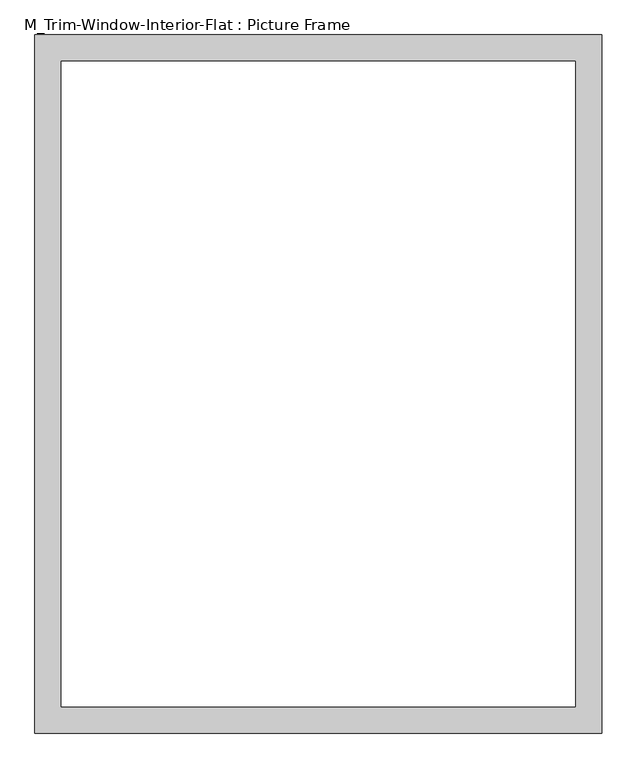
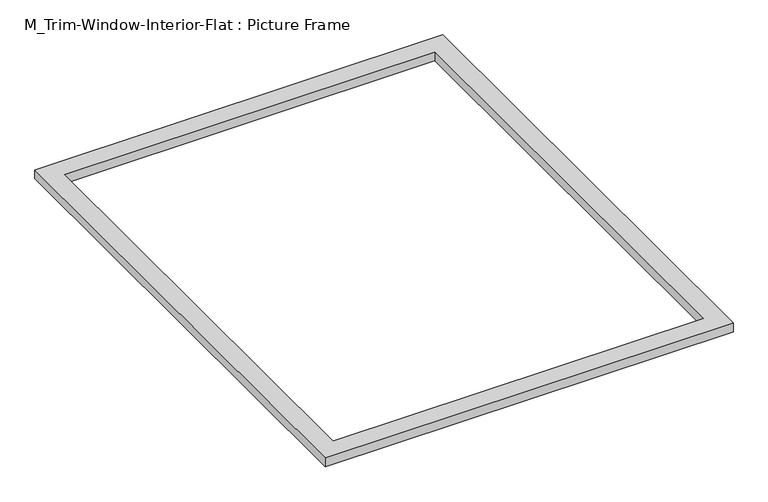
"""IFC4 building model written with IfcOpenShell, lengths in millimetres: proxy geometry, M_Trim-Window-Interior-Flat : Picture Frame."""

from ifc_helpers import new_model, si_unit, origin, origin_with_axes, place, context, project, spatial, polyline, outline, extrude, source, transform, mapped, element, save


def m_trim_window_interior_flat_picture_frame_5bf35ee4(model_context):
    return source(origin(), model_context, "Body", "SweptSolid", [
        extrude(outline(polyline([(647.3, 47.3), (647.3, -1547.3), (-647.3, -1547.3), (-647.3, 47.3), (647.3, 47.3)]), holes=[polyline([(587.3, -12.7), (-587.3, -12.7), (-587.3, -1487.3), (587.3, -1487.3), (587.3, -12.7)])]), origin_with_axes(), (0.0, 0.0, 1.0), 30.0),
    ])


if __name__ == "__main__":
    model = new_model("IFC4")
    model_context = context("Model", 3, world=origin())
    ifc_project = project(units=[si_unit("LENGTHUNIT", "METRE", prefix="MILLI")], contexts=[model_context])
    site = spatial("IfcSite", under=ifc_project)
    building = spatial("IfcBuilding", under=site)
    placement = place(None, origin())
    m_trim_window_interior_flat_picture_frame_shape = m_trim_window_interior_flat_picture_frame_5bf35ee4(model_context)
    element("IfcBuildingElementProxy", 1, Name="M_Trim-Window-Interior-Flat : Picture Frame", ObjectType="M_Trim-Window-Interior-Flat : Picture Frame", at=placement, inside=building, context=model_context, shape_type="MappedRepresentation", body=[
        mapped(m_trim_window_interior_flat_picture_frame_shape, transform((0.0, 0.0, 0.0), x_axis=(1.0, 0.0, 0.0), y_axis=(0.0, 1.0, 0.0), z_axis=(0.0, 0.0, 1.0))),
    ])
    save(model, "model.ifc")

# Revit data of these elements
# Type "M_Trim-Window-Interior-Flat : Picture Frame"
#   Trim Thickness_Picture Frame = 0.098425 ft
#   Trim Width = 0.19685 ft
#   Trim Thickness_with Sill = 0.065617 ft
#   Sill Thickness = 0.098425 ft
#   Opening Width [instance default] = 1.968504 ft
#   Opening Height [instance default] = 2.952756 ft
#   Default Elevation = 3.937008 ft
#   Sill = no
#   Picture Frame = yes
#   Trim Material [instance default] = none
# Element 1 (IfcBuildingElementProxy, "M_Trim-Window-Interior-Flat : Picture Frame")
#   Opening Width = 3.937008 ft
#   Opening Height = 4.92126 ft
#   Trim Material = Wood - Stained
#   Materials on its faces: "Wood - Stained"
# Materials
#   "Wood - Stained": class "Wood", colour RGB 224 178 126, transparency 0, Cost = 0
